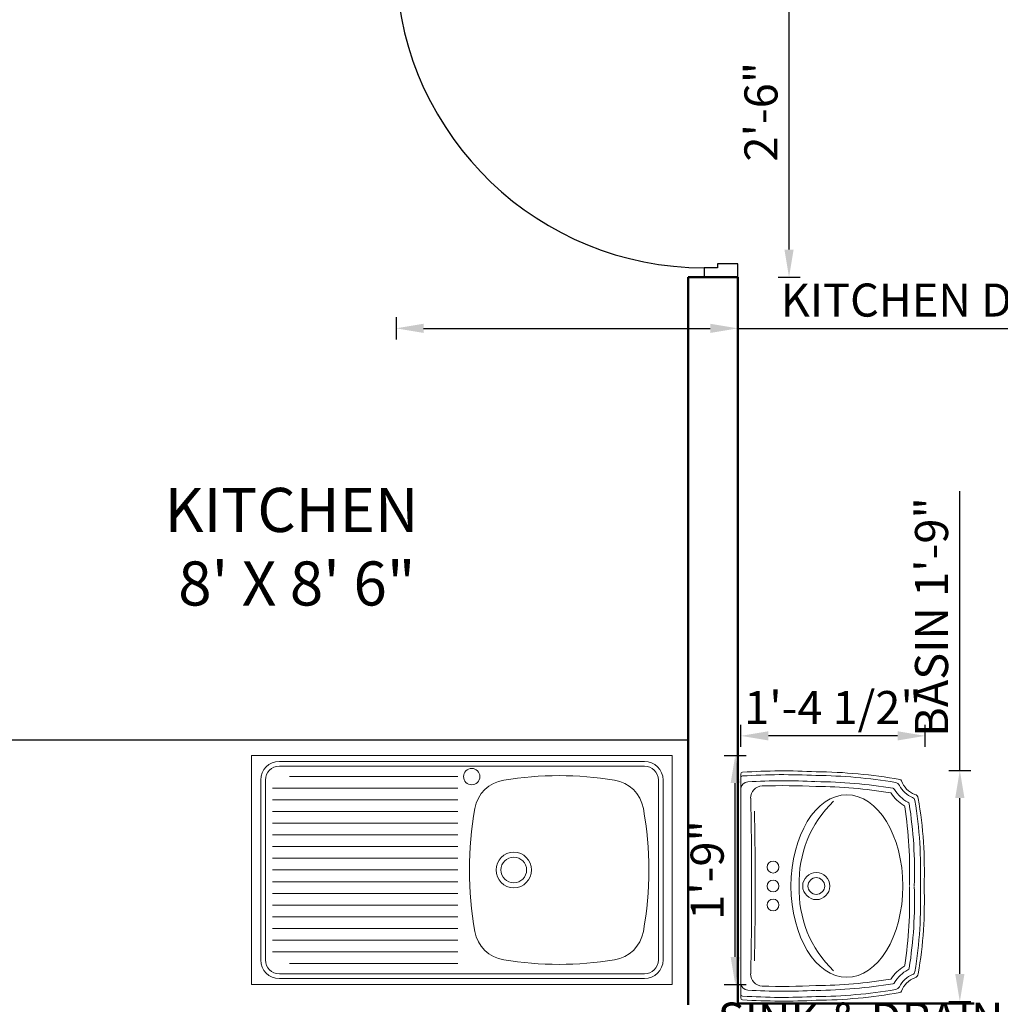
# Model space of a CAD drawing. Units: inches. Extents: x 1961 to 3038, y 800 to 1438.
# Tile 4 of 13: x 2666 to 2755, y 1058 to 1148. Entities that reach past the tile are written whole.
import ezdxf

# ---------------------------------------------------------------- set-up
doc = ezdxf.new("R2010")
doc.units = ezdxf.units.IN
for name, color, linetype, lineweight in [('A-ANNO-DIMS', 2, 'Continuous', 18), ('A-AREA-IDEN', 7, 'Continuous', 25), ('A-DOOR', 3, 'Continuous', 25), ('A-FLOR-CASE', 8, 'Continuous', 25), ('A-FLOR-FIXT', 9, 'Continuous', 18), ('A-WALL', 7, 'Continuous', 50)]:
    doc.layers.add(name, color=color, linetype=linetype, lineweight=lineweight)
doc.styles.get("Standard").update_dxf_attribs({"font": 'arial.ttf'})
doc.dimstyles.new('ISO-25', dxfattribs={"dimtxt": 3, "dimasz": 2.5, "dimexe": 1, "dimexo": 1, "dimtad": 1, "dimdec": 4, "dimlunit": 4, "dimtxsty": 'Standard', "dimcen": 2.5, "dimadec": 0, "dimazin": 0, "dimtfac": 1, "dimtdec": 4, "dimtmove": 0, "dimatfit": 3, "dimfxl": 1, "dimfxlon": 1, "dimarcsym": 0})

# ---------------------------------------------------------------- blocks, each defined once
blk = doc.blocks.new('door 26')
for p, q in [((2713.128, 1128.043), (2713.128, 1125.798)), ((2716.165, 1126.643), (2716.165, 1128.043)), ((2685.189, 1125.639), (2685.189, 1127.012)), ((2685.189, 1127.012), (2713.128, 1127.012)), ((2713.128, 1127.012), (2714.343, 1127.012)), ((2714.343, 1127.012), (2714.343, 1126.643)), ((2714.343, 1126.643), (2716.165, 1126.643)), ((2713.128, 1125.798), (2685.189, 1125.798))]:
    blk.add_line(p, q)
blk.add_lwpolyline([(2716.165, 1098.043), (2716.165, 1099.257), (2714.343, 1099.257), (2714.343, 1098.888), (2713.128, 1098.888), (2713.128, 1098.043)])
blk.add_arc((2713.128, 1126.854), 27.966, 182.48955, 270)
blk = doc.blocks.new('A$C55872771')
at = {"ltscale": 20}
for q in [(0.0084, 0.4917), (0.6091, 0.4917)]:
    blk.add_line((0.3087, 0.4917), q, dxfattribs=at)
for centre in [(0.2579, 0.4052), (0.3087, 0.4052), (0.3595, 0.4052)]:
    blk.add_circle(centre, 0.0159, dxfattribs=at)
for centre, radius, start, end in [((1.7227, 0.3777), 1.7227, 176.3626, 182.928), ((0.0084, 0.4867), 0.005, 90, 176.3626), ((1.7227, 0.3777), 1.7127, 176.3413, 182.928), ((0.0184, 0.4867), 0.005, 90, 176.3413), ((0.0491, 0.4717), 0.02, 90, 176.7861), ((0.5684, 0.4717), 0.02, 3.2139, 90), ((0.599, 0.4867), 0.005, 3.6587, 90), ((-1.1052, 0.3777), 1.7127, 357.072, 3.6587), ((0.6091, 0.4867), 0.005, 3.6374, 90), ((-1.1052, 0.3777), 1.7227, 357.072, 3.6374), ((1.7227, 0.3777), 1.6962, 176.7861, 182.928), ((0.0724, 0.4332), 0.032, 88.7903, 178.0749), ((0.3087, 11.6257), 11.1631, 268.79032, 270), ((0.3087, 11.6257), 11.1726, 268.97197, 270), ((0.3087, 11.6257), 11.1631, 270, 271.20968), ((0.3087, 11.6257), 11.1726, 270, 271.02803), ((0.5451, 0.4332), 0.032, 1.9251, 91.2097), ((-1.1052, 0.3777), 1.6962, 357.072, 3.2139), ((1.743, 0.3775), 1.7035, 178.0894, 182.9416), ((-1.1255, 0.3775), 1.7035, 357.0584, 1.9106), ((0.2983, 0.0346), 0.3007, 88.0093, 136.1344), ((0.3087, 0.2892), 0.0365, 90, 270), ((0.3192, 0.0346), 0.3007, 43.8656, 91.9907), ((0.3087, 0.2892), 0.0365, 270, 90), ((0.3087, 0.2892), 0.0225, 90, 270), ((0.3087, 0.2892), 0.0225, 270, 90), ((1.3508, 0.3007), 1.3486, 180.4656, 190.0418), ((1.3522, 0.3009), 1.34, 180.4547, 189.6069), ((1.3508, 0.3007), 1.3221, 180.4656, 189.4524), ((1.3508, 0.3007), 1.3091, 180.4656, 189.2524), ((-0.7333, 0.3007), 1.3091, 350.7476, 359.5344), ((-0.7333, 0.3007), 1.3221, 350.5476, 359.5344), ((-0.7333, 0.3007), 1.3386, 350.3906, 359.5344), ((-0.7333, 0.3007), 1.3486, 349.9582, 359.5344), ((0.0525, 0.0845), 0.006, 189.4524, 239.8947), ((0.0051, 0.0027), 0.0886, 27.3355, 59.8947), ((0.0617, 0.0907), 0.003, 189.2524, 237.2579), ((0.0051, 0.0027), 0.1016, 30.6701, 57.2579), ((0.6124, 0.0027), 0.1016, 122.7421, 149.3299), ((0.6124, 0.0027), 0.0886, 120.1053, 152.6645), ((0.5558, 0.0907), 0.003, 302.7421, 350.7476), ((0.5649, 0.0845), 0.006, 300.1053, 350.5476), ((0.0287, 0.0666), 0.006, 189.8911, 249.8861), ((0.0051, 0.0027), 0.0621, 21.454, 69.658), ((0.0457, 0.0797), 0.015, 189.6094, 242.1773), ((0.0051, 0.0027), 0.0721, 23.0692, 62.1773), ((0.0968, 0.0571), 0.005, 210.6701, 261.1326), ((0.5207, 0.0571), 0.005, 278.8674, 329.3299), ((0.6124, 0.0027), 0.0721, 117.8227, 156.9308), ((0.6124, 0.0027), 0.0621, 110.342, 158.546), ((0.5717, 0.0797), 0.015, 297.8227, 350.3906), ((0.5887, 0.0666), 0.006, 290.1139, 350.1089), ((0.0806, 0.0349), 0.01, 203.0692, 260.4945), ((0.0891, 0.0461), 0.006, 207.3355, 260.8302), ((0.2666, 1.1454), 1.1195, 260.8302, 272.1091), ((0.2666, 1.1454), 1.1065, 261.1326, 272.1091), ((0.3509, 1.1454), 1.1195, 267.8909, 279.1698), ((0.3509, 1.1454), 1.1065, 267.8909, 278.8674), ((0.5284, 0.0461), 0.006, 279.1698, 332.6645), ((0.5369, 0.0349), 0.01, 279.5055, 336.9308), ((0.0751, 0.0282), 0.0125, 192.82, 263.2226), ((0.2666, 1.1454), 1.146, 260.3058, 272.1091), ((0.2666, 1.1454), 1.136, 260.4945, 272.1091), ((0.3509, 1.1454), 1.146, 267.8909, 279.6942), ((0.3509, 1.1454), 1.136, 267.8909, 279.5055), ((0.5424, 0.0282), 0.0125, 276.7774, 347.18)]:
    blk.add_arc(centre, radius, start, end, dxfattribs=at)
at = {"ltscale": 20, "extrusion": (0, 0, -1)}
blk.add_ellipse((0.3087, 0.2072), major_axis=(-0.2447, 0), ratio=0.61287, start_param=-1.570796, end_param=1.570796, dxfattribs=at)
at = {"ltscale": 20}
blk.add_ellipse((0.3087, 0.2072), major_axis=(0.2447, 0), ratio=0.61287, start_param=-1.570796, end_param=1.570796, dxfattribs=at)
blk = doc.blocks.new('A$C0C3933DC')
for p, q in [((0, 490), (0, 0)), ((900, 490), (0, 490)), ((900, 0), (900, 490)), ((59.5, 477.5), (450, 477.5)), ((59.5, 467.5), (450, 467.5)), ((840.5, 477.5), (450, 477.5)), ((840.5, 467.5), (450, 467.5)), ((441, 445), (80.7, 445)), ((19.5, 52.5), (19.5, 437.5)), ((29.5, 52.5), (29.5, 437.5)), ((870.5, 52.5), (870.5, 437.5)), ((880.5, 52.5), (880.5, 437.5)), ((441, 420), (45, 420)), ((441, 395), (45, 395)), ((441, 370), (45, 370)), ((441, 345), (45, 345)), ((441, 320), (45, 320)), ((441, 295), (45, 295)), ((441, 270), (45, 270)), ((441, 245), (45, 245)), ((441, 220), (45, 220)), ((441, 195), (45, 195)), ((441, 170), (45, 170)), ((441, 145), (45, 145)), ((441, 120), (45, 120)), ((441, 95), (45, 95)), ((441, 70), (45, 70)), ((441, 45), (80.7, 45)), ((450, 22.5), (59.5, 22.5)), ((450, 22.5), (840.5, 22.5)), ((0, 0), (900, 0)), ((450, 12.5), (59.5, 12.5)), ((450, 12.5), (840.5, 12.5))]:
    blk.add_line(p, q)
for centre, radius in [((471, 445), 17.5), ((561, 245), 38), ((561, 245), 27.5)]:
    blk.add_circle(centre, radius)
for centre, radius, start, end in [((59.5, 437.5), 40, 90, 180), ((59.5, 437.5), 30, 90, 180), ((840.5, 437.5), 40, 0, 90), ((840.5, 437.5), 30, 0, 90), ((658, -303), 750, 80.9213, 99.0787), ((551.5, 363.5), 75, 99.0787, 169.8852), ((764.5, 363.5), 75, 10.1148, 80.9213), ((1216, 245), 750, 169.8852, 190.1148), ((100, 245), 750, 349.8852, 10.1148), ((551.5, 126.5), 75, 190.1148, 260.9213), ((764.5, 126.5), 75, 279.0787, 349.8852), ((59.5, 52.5), 40, 180, 270), ((59.5, 52.5), 30, 180, 270), ((658, 793), 750, 260.9213, 279.0787), ((840.5, 52.5), 30, 270, 0), ((840.5, 52.5), 40, 270, 0)]:
    blk.add_arc(centre, radius, start, end)
blk = doc.blocks.new('*D51')
at = {"layer": 'A-ANNO-DIMS', "color": 0, "lineweight": -2, "transparency": 16777216}
for p, q in [((2700.291, 1120.773), (2700.291, 1118.773)), ((2731.268, 1120.773), (2731.268, 1118.773)), ((2702.791, 1119.773), (2728.768, 1119.773)), ((2731.268, 1119.773), (2776.157, 1119.773))]:
    blk.add_line(p, q, dxfattribs=at)
at = {"layer": 'A-ANNO-DIMS', "color": 0, "transparency": 16777216}
for points in [[(2702.791, 1120.19), (2702.791, 1119.357), (2700.291, 1119.773)], [(2728.768, 1120.19), (2728.768, 1119.357), (2731.268, 1119.773)]]:
    blk.add_solid(points, dxfattribs=at)
at = {"layer": 'Defpoints', "color": 0, "transparency": 16777216}
for p in [(2700.291, 1124.42), (2731.268, 1124.42), (2731.268, 1119.773)]:
    blk.add_point(p, dxfattribs=at)
at = {"layer": 'A-ANNO-DIMS', "color": 0, "transparency": 16777216, "insert": (2754.962, 1121.95), "char_height": 3, "attachment_point": 5}
blk.add_mtext('KITCHEN DOOR 2\'-7"', dxfattribs=at)
blk = doc.blocks.new('*D52')
at = {"layer": 'A-ANNO-DIMS', "color": 0, "lineweight": -2, "transparency": 16777216}
for p, q in [((2734.915, 1154.42), (2736.915, 1154.42)), ((2735.915, 1126.92), (2735.915, 1151.92)), ((2734.915, 1124.42), (2736.915, 1124.42))]:
    blk.add_line(p, q, dxfattribs=at)
at = {"layer": 'A-ANNO-DIMS', "color": 0, "transparency": 16777216}
for points in [[(2735.498, 1151.92), (2736.331, 1151.92), (2735.915, 1154.42)], [(2735.498, 1126.92), (2736.331, 1126.92), (2735.915, 1124.42)]]:
    blk.add_solid(points, dxfattribs=at)
at = {"layer": 'Defpoints', "color": 0, "transparency": 16777216}
for p in [(2731.268, 1154.42), (2735.915, 1154.42), (2731.268, 1124.42)]:
    blk.add_point(p, dxfattribs=at)
at = {"layer": 'A-ANNO-DIMS', "color": 0, "transparency": 16777216, "insert": (2733.758, 1139.42), "char_height": 3, "attachment_point": 5, "rotation": 90}
blk.add_mtext('2\'-6"', dxfattribs=at)
blk = doc.blocks.new('*D59')
at = {"layer": 'A-ANNO-DIMS', "color": 0, "lineweight": -2, "transparency": 16777216}
for p, q in [((2751.397, 1079.68), (2751.397, 1105.013)), ((2750.397, 1079.68), (2752.397, 1079.68)), ((2751.397, 1061.228), (2751.397, 1077.18)), ((2750.397, 1058.728), (2752.397, 1058.728))]:
    blk.add_line(p, q, dxfattribs=at)
at = {"layer": 'A-ANNO-DIMS', "color": 0, "transparency": 16777216}
for points in [[(2750.98, 1077.18), (2751.814, 1077.18), (2751.397, 1079.68)], [(2750.98, 1061.228), (2751.814, 1061.228), (2751.397, 1058.728)]]:
    blk.add_solid(points, dxfattribs=at)
at = {"layer": 'Defpoints', "color": 0, "transparency": 16777216}
for p in [(2748.254, 1079.68), (2751.397, 1079.68), (2748.254, 1058.728)]:
    blk.add_point(p, dxfattribs=at)
at = {"layer": 'A-ANNO-DIMS', "color": 0, "transparency": 16777216, "insert": (2749.221, 1093.596), "char_height": 3, "attachment_point": 5, "rotation": 90}
blk.add_mtext('BASIN 1\'-9"', dxfattribs=at)
blk = doc.blocks.new('*D60')
at = {"layer": 'A-ANNO-DIMS', "color": 0, "lineweight": -2, "transparency": 16777216}
for p, q in [((2731.541, 1081.822), (2731.541, 1083.822)), ((2748.254, 1081.822), (2748.254, 1083.822)), ((2745.754, 1082.822), (2734.041, 1082.822))]:
    blk.add_line(p, q, dxfattribs=at)
at = {"layer": 'A-ANNO-DIMS', "color": 0, "transparency": 16777216}
for points in [[(2734.041, 1083.239), (2734.041, 1082.406), (2731.541, 1082.822)], [(2745.754, 1083.239), (2745.754, 1082.406), (2748.254, 1082.822)]]:
    blk.add_solid(points, dxfattribs=at)
at = {"layer": 'Defpoints', "color": 0, "transparency": 16777216}
for p in [(2731.541, 1082.822), (2731.541, 1079.68), (2748.254, 1079.68)]:
    blk.add_point(p, dxfattribs=at)
at = {"layer": 'A-ANNO-DIMS', "color": 0, "transparency": 16777216, "insert": (2739.898, 1084.998), "char_height": 3, "attachment_point": 5}
blk.add_mtext('1\'-4 1/2"', dxfattribs=at)
blk = doc.blocks.new('*D69')
at = {"layer": 'A-ANNO-DIMS', "color": 0, "lineweight": -2, "transparency": 16777216}
for p, q in [((2687.202, 1055.563), (2687.202, 1053.563)), ((2725.322, 1055.563), (2725.322, 1053.563)), ((2689.702, 1054.563), (2722.822, 1054.563)), ((2725.322, 1054.563), (2771.964, 1054.563))]:
    blk.add_line(p, q, dxfattribs=at)
at = {"layer": 'A-ANNO-DIMS', "color": 0, "transparency": 16777216}
for points in [[(2689.702, 1054.979), (2689.702, 1054.146), (2687.202, 1054.563)], [(2722.822, 1054.979), (2722.822, 1054.146), (2725.322, 1054.563)]]:
    blk.add_solid(points, dxfattribs=at)
at = {"layer": 'Defpoints', "color": 0, "transparency": 16777216}
for p in [(2687.202, 1060.281), (2725.322, 1060.281), (2725.322, 1054.563)]:
    blk.add_point(p, dxfattribs=at)
at = {"layer": 'A-ANNO-DIMS', "color": 0, "transparency": 16777216, "insert": (2749.893, 1056.748), "char_height": 3, "attachment_point": 5}
blk.add_mtext('SINK & DRAINER 3\'-2"', dxfattribs=at)
blk = doc.blocks.new('*D70')
at = {"layer": 'A-ANNO-DIMS', "color": 0, "lineweight": -2, "transparency": 16777216}
for p, q in [((2730.04, 1081.035), (2732.04, 1081.035)), ((2731.04, 1062.781), (2731.04, 1078.535)), ((2730.04, 1060.281), (2732.04, 1060.281))]:
    blk.add_line(p, q, dxfattribs=at)
at = {"layer": 'A-ANNO-DIMS', "color": 0, "transparency": 16777216}
for points in [[(2730.623, 1078.535), (2731.456, 1078.535), (2731.04, 1081.035)], [(2730.623, 1062.781), (2731.456, 1062.781), (2731.04, 1060.281)]]:
    blk.add_solid(points, dxfattribs=at)
at = {"layer": 'Defpoints', "color": 0, "transparency": 16777216}
for p in [(2725.322, 1081.035), (2731.04, 1081.035), (2725.322, 1060.281)]:
    blk.add_point(p, dxfattribs=at)
at = {"layer": 'A-ANNO-DIMS', "color": 0, "transparency": 16777216, "insert": (2728.883, 1070.658), "char_height": 3, "attachment_point": 5, "rotation": 90}
blk.add_mtext('1\'-9"', dxfattribs=at)

msp = doc.modelspace()

# ---------------------------------------------------------------- linework, layer by layer
at = {"layer": 'A-FLOR-CASE'}
msp.add_line((2726.76803, 1082.41975), (2654.76803, 1082.41975), dxfattribs=at)
at = {"layer": 'A-WALL'}
for p, q in [((2731.26803, 1124.41975), (2726.76803, 1124.41975)), ((2726.76803, 1124.41975), (2726.76803, 1058.41975)), ((2731.26803, 1124.41975), (2731.26803, 1058.41975)), ((2752.6978, 1058.53653), (2731.37674, 1058.53653))]:
    msp.add_line(p, q, dxfattribs=at)

# ---------------------------------------------------------------- block references
at = {"layer": 'A-DOOR'}
msp.add_blockref('door 26', (15.10265, 26.37719), dxfattribs=at)
at = {"layer": 'A-FLOR-FIXT', "xscale": 0.0423551022791598, "yscale": 0.0423551022791598, "zscale": 0.0423551022791598}
msp.add_blockref('A$C0C3933DC', (2687.20225, 1060.28053), dxfattribs=at)
at = {"layer": 'A-FLOR-FIXT', "xscale": 33.8044925571632, "yscale": 33.8044925571632, "zscale": 33.8044925571632, "rotation": 90}
msp.add_blockref('A$C55872771', (2748.16278, 1058.76714), dxfattribs=at)

# ---------------------------------------------------------------- texts
at = {"layer": 'A-AREA-IDEN', "insert": (2679.32463, 1105.30625), "char_height": 4, "attachment_point": 1}
msp.add_mtext_dynamic_manual_height_columns('{\\fTimes New Roman|b1|i0|c0|p18;KITCHEN\\P 8\' X 8\' 6"}', width=33.1080891, gutter_width=12.5, heights=[0], dxfattribs=at)

# ---------------------------------------------------------------- dimensions: what is measured, and where the dimension line sits
at = {"layer": 'A-ANNO-DIMS'}
for base, p1, p2, angle, picture, middle in [((2735.91454, 1154.41975), (2731.26803, 1124.41975), (2731.26803, 1154.41975), 90, '*D52', (2733.75783, 1139.41975)), ((2731.54128, 1082.82225), (2748.25418, 1079.67957), (2731.54128, 1079.67957), 180, '*D60', (2739.89773, 1084.9984)), ((2731.03978, 1081.03453), (2725.32185, 1060.28053), (2725.32185, 1081.03453), 90, '*D70', (2728.88307, 1070.65753))]:
    dim = msp.add_linear_dim(base=base, p1=p1, p2=p2, angle=angle, dimstyle='ISO-25', override={"dimdec": 1, "dimlfac": 1, "dimrnd": 0, "dimzin": 1, "dimdsep": 46, "dimlunit": 4, "dimfrac": 2}, dxfattribs=at)
    dim.commit()
    dim.dimension.update_dxf_attribs({"geometry": picture, "text_midpoint": middle})
for base, p1, p2, text, picture, middle in [((2731.26803, 1119.77324), (2700.29129, 1124.41975), (2731.26803, 1124.41975), 'KITCHEN DOOR <>', '*D51', (2754.96227, 1121.95042)), ((2725.32185, 1054.56259), (2687.20225, 1060.28053), (2725.32185, 1060.28053), 'SINK & DRAINER <>', '*D69', (2749.89296, 1056.74796))]:
    dim = msp.add_linear_dim(base=base, p1=p1, p2=p2, text=text, dimstyle='ISO-25', override={"dimdec": 1, "dimlfac": 1, "dimrnd": 0, "dimzin": 1, "dimdsep": 46, "dimlunit": 4, "dimfrac": 2}, dxfattribs=at)
    dim.commit()
    dim.dimension.update_dxf_attribs({"geometry": picture, "text_midpoint": middle})
dim = msp.add_linear_dim(base=(2751.39685, 1079.67957), p1=(2748.25418, 1058.7284), p2=(2748.25418, 1079.67957), angle=90, text='BASIN <>', dimstyle='ISO-25', override={"dimdec": 1, "dimlfac": 1, "dimrnd": 0, "dimzin": 1, "dimdsep": 46, "dimlunit": 4, "dimfrac": 2}, dxfattribs=at)
dim.commit()
dim.dimension.update_dxf_attribs({"geometry": '*D59', "text_midpoint": (2749.22069, 1093.59618)})

doc.saveas('drawing.dxf')
